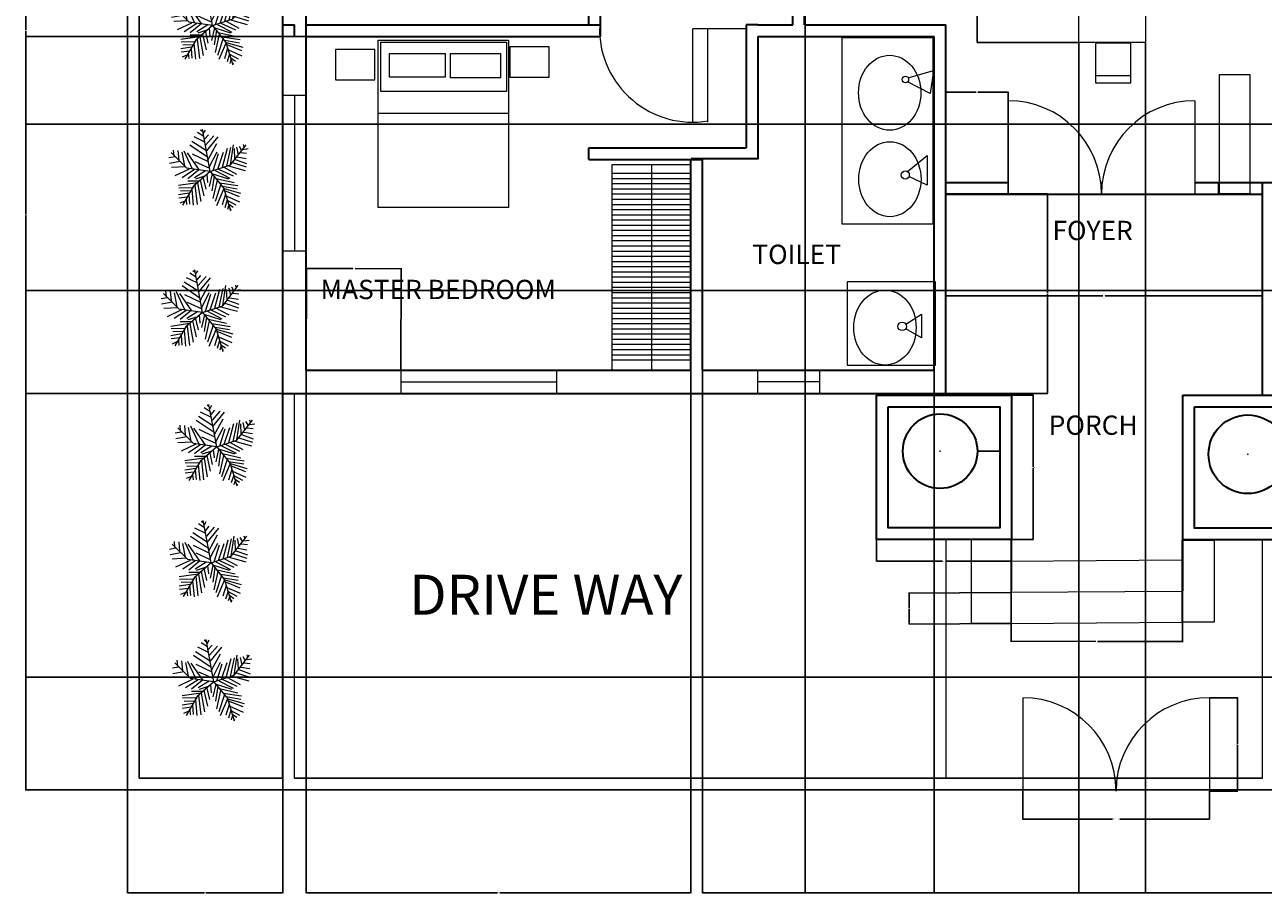
# Model space of a CAD drawing. Units: inches. Extents: x -86 to 773, y -188 to 560.
# Tile 1 of 6: x -86 to 392, y -188 to 147. Entities that reach past the tile are written whole.
import ezdxf

# ---------------------------------------------------------------- set-up
doc = ezdxf.new("R2010")
doc.units = ezdxf.units.IN
doc.header["$MEASUREMENT"] = 0
for name, color, linetype, lineweight in [('A-ANNO-DIMS', 2, 'Continuous', 18), ('A-AREA-IDEN', 7, 'Continuous', 25), ('A-COLS', 7, 'Continuous', 35), ('A-DOOR', 7, 'Continuous', 18), ('A-FLOR-FIXT', 8, 'Continuous', 18), ('A-FLOR-STRS', 7, 'Continuous', 18), ('A-FURN', 8, 'Continuous', 18), ('A-FURN-PATT', 8, 'Continuous', 9), ('A-GLAZ', 7, 'Continuous', 18), ('A-WALL', 7, 'Continuous', 35), ('C-PROP', 7, 'Continuous', 25), ('L-HRDS', 7, 'Continuous', 18), ('L-PLNT-TREE', 8, 'Continuous', 9)]:
    doc.layers.add(name, color=color, linetype=linetype, lineweight=lineweight)
doc.styles.get("Standard").update_dxf_attribs({"font": 'arial.ttf'})
doc.dimstyles.get("Standard").update_dxf_attribs({"dimtxt": 0.18, "dimasz": 0.18, "dimexe": 0.18, "dimexo": 0.0625, "dimgap": 0.09, "dimtad": 0, "dimtih": 1, "dimtoh": 1, "dimdec": 4, "dimzin": 0, "dimdsep": 46, "dimtxsty": 'Standard', "dimcen": 0.09, "dimadec": 0, "dimazin": 0, "dimtfac": 1, "dimtdec": 4, "dimtofl": 0, "dimtmove": 0, "dimatfit": 3, "dimfxl": 1, "dimtolj": 1, "dimtzin": 0, "dimarcsym": 0})

# ---------------------------------------------------------------- blocks, each defined once
blk = doc.blocks.new('Trees - Metric')
for p, q in [((-221.9198, 1197.3052), (-433.5526, 1338.8594)), ((-258.7244, 1362.456), (-332.3336, 1421.4348)), ((0, 0), (-266.7, 1447.8)), ((-231.1146, 1315.2628), (-166.7002, 1421.4348)), ((-93.091, 489.5342), (-700.3796, 902.3858)), ((-129.8956, 713.6638), (-626.7704, 1032.1544)), ((-185.1152, 1008.5578), (-553.1612, 1185.4942)), ((-194.31, 1102.9442), (-65.4812, 1256.284)), ((-148.3106, 914.1968), (118.5418, 1220.9018)), ((-129.8956, 701.8528), (265.7602, 1185.4942)), ((-74.7014, 418.7444), (219.7608, 961.39)), ((685.8, 228.6), (1219.2, 914.4)), ((689.0258, 230.0224), (790.2448, 914.1968)), ((983.4626, 867.0036), (1066.2666, 725.4494)), ((1121.4862, 925.9824), (1149.0706, 831.6214)), ((-1206.4492, 501.3198), (-1418.082, 465.9376)), ((-800.1, 114.3), (-1333.5, 647.7)), ((-1234.059, 536.7274), (-1252.4486, 737.2604)), ((-1105.2302, 725.4494), (-1077.6458, 395.1732)), ((-976.4268, 666.4706), (-884.4026, 194.6402)), ((-902.8176, 713.6638), (-617.5756, 100.2538)), ((-369.1382, 53.086), (-783.1836, 642.874)), ((-617.5756, 607.4918), (-74.7014, 347.98)), ((-28.6766, 171.0436), (228.9556, 678.2816)), ((100.1268, 41.275), (284.1498, 619.2774)), ((256.5654, 88.4682), (449.7832, 666.4706)), ((412.9786, 147.447), (587.8068, 796.2392)), ((560.197, 182.8292), (698.2206, 819.8358)), ((808.6344, 784.4282), (827.0494, 418.7444)), ((891.4384, 831.6214), (946.658, 572.1096)), ((919.0482, 501.3198), (1222.6798, 454.152)), ((1029.462, 654.685), (1241.0948, 631.0884)), ((1112.2914, 760.8316), (1296.3144, 784.4282)), ((-1031.621, 347.98), (-1399.667, 277.1902)), ((-847.598, 159.2326), (-1326.0578, 135.636)), ((-718.7946, 88.4682), (-1215.644, -147.447)), ((-543.9664, 76.6572), (-967.2066, -206.4512)), ((0, 0), (-800.1, 114.3)), ((-405.9428, 53.086), (-764.794, -241.8334)), ((0, 0), (-571.5, -495.3)), ((-166.7002, 29.4894), (-543.9664, -206.4512)), ((-525.5514, 347.98), (-28.6766, 123.8504)), ((0, 0), (685.8, 228.6)), ((0, 0), (457.2, -571.5)), ((164.5412, 41.275), (661.416, -218.2368)), ((284.1498, 88.4682), (781.0246, -147.447)), ((458.978, 147.447), (891.4384, -88.4682)), ((615.4166, 194.6402), (1185.8752, 41.275)), ((753.4148, 312.5978), (1222.6798, 159.2326)), ((845.439, 418.7444), (1241.0948, 277.1902)), ((-442.7474, -383.3876), (-1086.8406, -477.7486)), ((-387.5278, -324.4088), (-764.794, -324.4088)), ((-166.7002, -147.447), (-507.1618, -253.619)), ((-433.5526, -383.3876), (-323.1134, -1020.3688)), ((-341.5284, -289.0012), (-221.9198, -831.6214)), ((-240.3094, -218.2368), (-157.5054, -595.7062)), ((-120.7008, -88.4682), (-93.091, -371.5766)), ((63.3222, -76.6826), (-37.8714, -513.1308)), ((44.9326, -64.897), (615.4166, -241.8334)), ((127.7366, -159.258), (54.1274, -654.685)), ((228.9556, -289.0012), (90.932, -914.1968)), ((192.151, -230.0224), (817.8292, -371.5766)), ((311.7596, -383.3876), (937.4378, -477.7486)), ((-718.7946, -737.2604), (-1086.8406, -796.2392)), ((-617.5756, -548.5384), (-1077.6458, -560.324)), ((-681.9646, -666.496), (-1022.4262, -654.685)), ((-571.5, -495.3), (-952.5, -1143)), ((-737.1842, -784.4536), (-709.5744, -1114.7298)), ((-635.9652, -607.5172), (-580.771, -1150.1374)), ((-525.5514, -465.963), (-451.9422, -1126.5408)), ((357.759, -430.5554), (164.5412, -1020.3688)), ((458.978, -572.1096), (210.5406, -1161.923)), ((514.1976, -772.6426), (403.7838, -1138.3264)), ((412.9786, -501.3452), (919.0482, -583.9206)), ((457.2, -571.5), (685.8, -1333.5)), ((468.1982, -572.1096), (1029.462, -737.2604)), ((486.5878, -642.8994), (983.4626, -843.4324)), ((541.8074, -831.6214), (992.6574, -1032.1544)), ((-783.1836, -867.029), (-1077.6458, -902.4112)), ((-875.2078, -1008.5832), (-1040.8412, -1079.3476)), ((-829.2084, -937.7934), (-810.7934, -1126.5408)), ((578.612, -961.39), (495.7826, -1232.7128)), ((578.612, -973.1756), (873.0488, -1138.3264)), ((624.6114, -1161.923), (587.8068, -1291.6916)), ((624.6114, -1102.9442), (781.0246, -1209.1162)), ((679.8056, -1268.095), (716.6102, -1291.6916))]:
    blk.add_line(p, q)
blk = doc.blocks.new('BED-DOUBLE-NIGHTSTANDS')
blk.add_line((16.69, 36.48), (66.76, 36.48))
for points in [[(16.43, 64.62), (66.76, 64.62), (66.76, 0), (16.43, 0)], [(17.47, 63.83), (65.98, 63.83), (65.98, 44.81), (17.47, 44.81)], [(15.13, 60.97), (0, 60.97), (0, 49.24), (15.13, 49.24)], [(20.86, 59.41), (42.25, 59.41), (42.25, 50.29), (20.86, 50.29)], [(44.34, 59.41), (63.63, 59.41), (63.63, 50.03), (44.34, 50.03)], [(82.41, 62.01), (67.29, 62.01), (67.29, 50.29), (82.41, 50.29)]]:
    blk.add_lwpolyline(points, close=True)
blk = doc.blocks.new('DOOR-DOUBLE-72')
for p, q in [((0, 36), (0, 0)), ((72, 36), (72, 0))]:
    blk.add_line(p, q)
for centre, start, end in [((0, 0), 0, 90), ((72, 0), 90, 180)]:
    blk.add_arc(centre, 36, start, end)
blk = doc.blocks.new('WIN-60-W9')
for p, q in [((0, 60), (9, 60)), ((4.5, 60), (4.5, 0)), ((0, 0), (9, 0))]:
    blk.add_line(p, q)
blk = doc.blocks.new('WIN-24-W9')
for p, q in [((0, 9), (0, 0)), ((24, 9), (24, 0)), ((24, 4.5), (0, 4.5))]:
    blk.add_line(p, q)
blk = doc.blocks.new('DINING-CHAIR')
blk.add_line((0, 12.55), (13.8, 12.55))
blk.add_lwpolyline([(0.02, 0), (13.65, 0), (13.65, 15.22), (0.02, 15.22)], close=True)
blk = doc.blocks.new('BASIN-TAP')
blk.add_lwpolyline([(3.11, 5.27), (9.09, 9.11), (9.09, 0), (3.06, 3.55)])
blk.add_circle((1.66, 4.45), 1.66)
blk = doc.blocks.new('PORCH-COLUMN-PLINTH')
for points in [[(0, 55.74), (51.99, 55.74), (51.99, 0), (0, 0)], [(4.5, 51.24), (47.49, 51.24), (47.49, 4.5), (4.5, 4.5)]]:
    blk.add_lwpolyline(points, close=True)
blk = doc.blocks.new('*D33')
at = {"layer": 'A-ANNO-DIMS', "color": 0, "lineweight": -2, "transparency": 16777216}
for p, q in [((299.01, -148.39), (299.01, -159.31)), ((371.01, -148.39), (371.01, -159.31)), ((299.19, -159.13), (333.59, -159.13)), ((370.83, -159.13), (336.44, -159.13))]:
    blk.add_line(p, q, dxfattribs=at)
at = {"layer": 'A-ANNO-DIMS', "color": 0, "transparency": 16777216}
for points in [[(299.19, -159.1), (299.19, -159.16), (299.01, -159.13)], [(370.83, -159.1), (370.83, -159.16), (371.01, -159.13)]]:
    blk.add_solid(points, dxfattribs=at)
at = {"layer": 'Defpoints', "color": 0, "transparency": 16777216}
for p in [(299.01, -148.33), (371.01, -148.33), (371.01, -159.13)]:
    blk.add_point(p, dxfattribs=at)
at = {"layer": 'A-ANNO-DIMS', "color": 0, "transparency": 16777216, "insert": (335.01, -159.13), "char_height": 0.18, "attachment_point": 5}
blk.add_mtext('\\A1;DOUBLE LEAF 72 TYP.', dxfattribs=at)
blk = doc.blocks.new('*D34')
at = {"layer": 'A-ANNO-DIMS', "color": 0, "lineweight": -2, "transparency": 16777216}
for p, q in [((371.08, -112.33), (381.99, -112.33)), ((381.81, -112.51), (381.81, -130.15)), ((381.81, -148.15), (381.81, -130.51)), ((371.08, -148.33), (381.99, -148.33))]:
    blk.add_line(p, q, dxfattribs=at)
at = {"layer": 'A-ANNO-DIMS', "color": 0, "transparency": 16777216}
for points in [[(381.78, -112.51), (381.84, -112.51), (381.81, -112.33)], [(381.78, -148.15), (381.84, -148.15), (381.81, -148.33)]]:
    blk.add_solid(points, dxfattribs=at)
at = {"layer": 'Defpoints', "color": 0, "transparency": 16777216}
for p in [(371.01, -112.33), (381.81, -112.33), (371.01, -148.33)]:
    blk.add_point(p, dxfattribs=at)
at = {"layer": 'A-ANNO-DIMS', "color": 0, "transparency": 16777216, "insert": (381.81, -130.33), "char_height": 0.18, "attachment_point": 5}
blk.add_mtext('\\A1;36 TYP.', dxfattribs=at)
blk = doc.blocks.new('*D43')
at = {"layer": 'A-ANNO-DIMS', "color": 0, "lineweight": -2, "transparency": 16777216}
for p, q in [((294.66, 4.44), (303.14, 4.44)), ((302.96, 4.26), (302.96, -23.25)), ((302.96, -51.12), (302.96, -23.61)), ((294.66, -51.3), (303.14, -51.3))]:
    blk.add_line(p, q, dxfattribs=at)
at = {"layer": 'A-ANNO-DIMS', "color": 0, "transparency": 16777216}
for points in [[(302.93, 4.26), (302.99, 4.26), (302.96, 4.44)], [(302.93, -51.12), (302.99, -51.12), (302.96, -51.3)]]:
    blk.add_solid(points, dxfattribs=at)
at = {"layer": 'Defpoints', "color": 0, "transparency": 16777216}
for p in [(294.6, 4.44), (302.96, 4.44), (294.6, -51.3)]:
    blk.add_point(p, dxfattribs=at)
at = {"layer": 'A-ANNO-DIMS', "color": 0, "transparency": 16777216, "insert": (302.96, -23.43), "char_height": 0.18, "attachment_point": 5}
blk.add_mtext('\\A1;PLINTH 56 TYP.', dxfattribs=at)
blk = doc.blocks.new('*D44')
at = {"layer": 'A-ANNO-DIMS', "color": 0, "lineweight": -2, "transparency": 16777216}
for p, q in [((242.61, -51.36), (242.61, -59.84)), ((294.6, -51.36), (294.6, -59.84)), ((242.79, -59.66), (268.07, -59.66)), ((294.42, -59.66), (269.13, -59.66))]:
    blk.add_line(p, q, dxfattribs=at)
at = {"layer": 'A-ANNO-DIMS', "color": 0, "transparency": 16777216}
for points in [[(242.79, -59.63), (242.79, -59.69), (242.61, -59.66)], [(294.42, -59.63), (294.42, -59.69), (294.6, -59.66)]]:
    blk.add_solid(points, dxfattribs=at)
at = {"layer": 'Defpoints', "color": 0, "transparency": 16777216}
for p in [(242.61, -51.3), (294.6, -51.3), (294.6, -59.66)]:
    blk.add_point(p, dxfattribs=at)
at = {"layer": 'A-ANNO-DIMS', "color": 0, "transparency": 16777216, "insert": (268.6, -59.66), "char_height": 0.18, "attachment_point": 5}
blk.add_mtext('\\A1;52 TYP.', dxfattribs=at)
blk = doc.blocks.new('*D47')
at = {"layer": 'A-ANNO-DIMS', "color": 0, "lineweight": -2, "transparency": 16777216}
for p, q in [((-46.55, -147.98), (-46.55, -187.76)), ((13.45, -143.48), (13.45, -187.76)), ((-46.37, -187.58), (-16.77, -187.58)), ((13.27, -187.58), (-16.33, -187.58))]:
    blk.add_line(p, q, dxfattribs=at)
at = {"layer": 'A-ANNO-DIMS', "color": 0, "transparency": 16777216}
for points in [[(-46.37, -187.55), (-46.37, -187.61), (-46.55, -187.58)], [(13.27, -187.55), (13.27, -187.61), (13.45, -187.58)]]:
    blk.add_solid(points, dxfattribs=at)
at = {"layer": 'Defpoints', "color": 0, "transparency": 16777216}
for p in [(-46.55, -147.92), (13.45, -143.42), (13.45, -187.58)]:
    blk.add_point(p, dxfattribs=at)
at = {"layer": 'A-ANNO-DIMS', "color": 0, "transparency": 16777216, "insert": (-16.55, -187.58), "char_height": 0.18, "attachment_point": 5}
blk.add_mtext('\\A1;60', dxfattribs=at)
blk = doc.blocks.new('*D49')
at = {"layer": 'A-ANNO-DIMS', "color": 0, "lineweight": -2, "transparency": 16777216}
for p, q in [((13.39, 5.02), (-85.98, 5.02)), ((-85.8, 4.84), (-85.8, -71.27)), ((-85.8, -147.74), (-85.8, -71.63)), ((-46.61, -147.92), (-85.98, -147.92))]:
    blk.add_line(p, q, dxfattribs=at)
at = {"layer": 'A-ANNO-DIMS', "color": 0, "transparency": 16777216}
for points in [[(-85.83, 4.84), (-85.77, 4.84), (-85.8, 5.02)], [(-85.83, -147.74), (-85.77, -147.74), (-85.8, -147.92)]]:
    blk.add_solid(points, dxfattribs=at)
at = {"layer": 'Defpoints', "color": 0, "transparency": 16777216}
for p in [(-85.8, 5.02), (13.45, 5.02), (-46.55, -147.92)]:
    blk.add_point(p, dxfattribs=at)
at = {"layer": 'A-ANNO-DIMS', "color": 0, "transparency": 16777216, "insert": (-85.8, -71.45), "char_height": 0.18, "attachment_point": 5}
blk.add_mtext('\\A1;152.94', dxfattribs=at)
blk = doc.blocks.new('*D50')
at = {"layer": 'A-ANNO-DIMS', "color": 0, "lineweight": -2, "transparency": 16777216}
for p, q in [((22.39, 142.78), (-85.98, 142.78)), ((-85.8, 142.6), (-85.8, 74.08)), ((-85.8, 5.2), (-85.8, 73.72)), ((13.39, 5.02), (-85.98, 5.02))]:
    blk.add_line(p, q, dxfattribs=at)
at = {"layer": 'A-ANNO-DIMS', "color": 0, "transparency": 16777216}
for points in [[(-85.83, 142.6), (-85.77, 142.6), (-85.8, 142.78)], [(-85.83, 5.2), (-85.77, 5.2), (-85.8, 5.02)]]:
    blk.add_solid(points, dxfattribs=at)
at = {"layer": 'Defpoints', "color": 0, "transparency": 16777216}
for p in [(-85.8, 142.78), (22.45, 142.78), (13.45, 5.02)]:
    blk.add_point(p, dxfattribs=at)
at = {"layer": 'A-ANNO-DIMS', "color": 0, "transparency": 16777216, "insert": (-85.8, 73.9), "char_height": 0.18, "attachment_point": 5}
blk.add_mtext('\\A1;137.76', dxfattribs=at)
blk = doc.blocks.new('*D53')
at = {"layer": 'A-ANNO-DIMS', "color": 0, "lineweight": -2, "transparency": 16777216}
for p, q in [((623.74, 44.83), (-85.98, 44.83)), ((-85.8, 44.65), (-85.8, -29.62)), ((-85.8, -104.26), (-85.8, -29.99)), ((623.93, -104.44), (-85.98, -104.44))]:
    blk.add_line(p, q, dxfattribs=at)
at = {"layer": 'A-ANNO-DIMS', "color": 0, "transparency": 16777216}
for points in [[(-85.83, 44.65), (-85.77, 44.65), (-85.8, 44.83)], [(-85.83, -104.26), (-85.77, -104.26), (-85.8, -104.44)]]:
    blk.add_solid(points, dxfattribs=at)
at = {"layer": 'Defpoints', "color": 0, "transparency": 16777216}
for p in [(623.81, 44.83), (-85.8, -104.44), (623.99, -104.44)]:
    blk.add_point(p, dxfattribs=at)
at = {"layer": 'A-ANNO-DIMS', "color": 0, "transparency": 16777216, "insert": (-85.8, -29.81), "char_height": 0.18, "attachment_point": 5}
blk.add_mtext('\\A1;149.27', dxfattribs=at)
blk = doc.blocks.new('*D63')
at = {"layer": 'A-ANNO-DIMS', "color": 0, "lineweight": -2, "transparency": 16777216}
for p, q in [((22.45, 13.96), (22.45, -187.76)), ((170.89, 13.96), (170.89, -187.76)), ((22.63, -187.58), (96.22, -187.58)), ((170.71, -187.58), (97.13, -187.58))]:
    blk.add_line(p, q, dxfattribs=at)
at = {"layer": 'A-ANNO-DIMS', "color": 0, "transparency": 16777216}
for points in [[(22.63, -187.55), (22.63, -187.61), (22.45, -187.58)], [(170.71, -187.55), (170.71, -187.61), (170.89, -187.58)]]:
    blk.add_solid(points, dxfattribs=at)
at = {"layer": 'Defpoints', "color": 0, "transparency": 16777216}
for p in [(22.45, 14.02), (170.89, 14.02), (170.89, -187.58)]:
    blk.add_point(p, dxfattribs=at)
at = {"layer": 'A-ANNO-DIMS', "color": 0, "transparency": 16777216, "insert": (96.67, -187.58), "char_height": 0.18, "attachment_point": 5}
blk.add_mtext('\\A1;148.44', dxfattribs=at)
blk = doc.blocks.new('*D64')
at = {"layer": 'A-ANNO-DIMS', "color": 0, "lineweight": -2, "transparency": 16777216}
for p, q in [((175.39, 13.96), (175.39, -187.76)), ((264.79, 13.96), (264.79, -187.76)), ((175.57, -187.58), (219.77, -187.58)), ((264.61, -187.58), (220.42, -187.58))]:
    blk.add_line(p, q, dxfattribs=at)
at = {"layer": 'A-ANNO-DIMS', "color": 0, "transparency": 16777216}
for points in [[(175.57, -187.55), (175.57, -187.61), (175.39, -187.58)], [(264.61, -187.55), (264.61, -187.61), (264.79, -187.58)]]:
    blk.add_solid(points, dxfattribs=at)
at = {"layer": 'Defpoints', "color": 0, "transparency": 16777216}
for p in [(175.39, 14.02), (264.79, 14.02), (264.79, -187.58)]:
    blk.add_point(p, dxfattribs=at)
at = {"layer": 'A-ANNO-DIMS', "color": 0, "transparency": 16777216, "insert": (220.09, -187.58), "char_height": 0.18, "attachment_point": 5}
blk.add_mtext('\\A1;89.4', dxfattribs=at)
blk = doc.blocks.new('*D65')
at = {"layer": 'A-ANNO-DIMS', "color": 0, "lineweight": -2, "transparency": 16777216}
for p, q in [((446.53, 366.45), (446.53, -187.76)), ((215.06, 361.95), (215.06, -187.76)), ((215.24, -187.58), (330.33, -187.58)), ((446.35, -187.58), (331.26, -187.58))]:
    blk.add_line(p, q, dxfattribs=at)
at = {"layer": 'A-ANNO-DIMS', "color": 0, "transparency": 16777216}
for points in [[(215.24, -187.55), (215.24, -187.61), (215.06, -187.58)], [(446.35, -187.55), (446.35, -187.61), (446.53, -187.58)]]:
    blk.add_solid(points, dxfattribs=at)
at = {"layer": 'Defpoints', "color": 0, "transparency": 16777216}
for p in [(446.53, 366.52), (215.06, 362.02), (446.53, -187.58)]:
    blk.add_point(p, dxfattribs=at)
at = {"layer": 'A-ANNO-DIMS', "color": 0, "transparency": 16777216, "insert": (330.8, -187.58), "char_height": 0.18, "attachment_point": 5}
blk.add_mtext('\\A1;231.47', dxfattribs=at)
blk = doc.blocks.new('*D66')
at = {"layer": 'A-ANNO-DIMS', "color": 0, "lineweight": -2, "transparency": 16777216}
for p, q in [((269.29, 81.93), (269.29, 42.57)), ((391.47, 81.93), (391.47, 42.57)), ((269.47, 42.75), (329.92, 42.75)), ((391.29, 42.75), (330.83, 42.75))]:
    blk.add_line(p, q, dxfattribs=at)
at = {"layer": 'A-ANNO-DIMS', "color": 0, "transparency": 16777216}
for points in [[(269.47, 42.78), (269.47, 42.72), (269.29, 42.75)], [(391.29, 42.78), (391.29, 42.72), (391.47, 42.75)]]:
    blk.add_solid(points, dxfattribs=at)
at = {"layer": 'Defpoints', "color": 0, "transparency": 16777216}
for p in [(269.29, 82), (391.47, 82), (269.29, 42.75)]:
    blk.add_point(p, dxfattribs=at)
at = {"layer": 'A-ANNO-DIMS', "color": 0, "transparency": 16777216, "insert": (330.38, 42.75), "char_height": 0.18, "attachment_point": 5}
blk.add_mtext('\\A1;122.17', dxfattribs=at)
blk = doc.blocks.new('*D73')
at = {"layer": 'A-ANNO-DIMS', "color": 0, "lineweight": -2, "transparency": 16777216}
for p, q in [((577.4, 181.27), (-85.98, 181.27)), ((-85.8, 181.09), (-85.8, 145.29)), ((-85.8, 109.12), (-85.8, 144.92)), ((577.4, 108.94), (-85.98, 108.94))]:
    blk.add_line(p, q, dxfattribs=at)
at = {"layer": 'A-ANNO-DIMS', "color": 0, "transparency": 16777216}
for points in [[(-85.83, 181.09), (-85.77, 181.09), (-85.8, 181.27)], [(-85.83, 109.12), (-85.77, 109.12), (-85.8, 108.94)]]:
    blk.add_solid(points, dxfattribs=at)
at = {"layer": 'Defpoints', "color": 0, "transparency": 16777216}
for p in [(-85.8, 181.27), (577.46, 181.27), (577.46, 108.94)]:
    blk.add_point(p, dxfattribs=at)
at = {"layer": 'A-ANNO-DIMS', "color": 0, "transparency": 16777216, "insert": (-85.8, 145.11), "char_height": 0.18, "attachment_point": 5}
blk.add_mtext('\\A1;72.33', dxfattribs=at)
blk = doc.blocks.new('*D77')
at = {"layer": 'A-ANNO-DIMS', "color": 0, "lineweight": -2, "transparency": 16777216}
for p, q in [((320.69, 140.33), (320.69, -187.76)), ((346.35, 140.33), (346.35, -187.76)), ((320.87, -187.58), (333.13, -187.58)), ((346.17, -187.58), (333.92, -187.58))]:
    blk.add_line(p, q, dxfattribs=at)
at = {"layer": 'A-ANNO-DIMS', "color": 0, "transparency": 16777216}
for points in [[(320.87, -187.55), (320.87, -187.61), (320.69, -187.58)], [(346.17, -187.55), (346.17, -187.61), (346.35, -187.58)]]:
    blk.add_solid(points, dxfattribs=at)
at = {"layer": 'Defpoints', "color": 0, "transparency": 16777216}
for p in [(320.69, 140.39), (346.35, 140.39), (346.35, -187.58)]:
    blk.add_point(p, dxfattribs=at)
at = {"layer": 'A-ANNO-DIMS', "color": 0, "transparency": 16777216, "insert": (333.52, -187.58), "char_height": 0.18, "attachment_point": 5}
blk.add_mtext('\\A1;25.66', dxfattribs=at)
blk = doc.blocks.new('*D78')
at = {"layer": 'A-ANNO-DIMS', "color": 0, "lineweight": -2, "transparency": 16777216}
for p, q in [((320.63, 194.07), (281.26, 194.07)), ((281.44, 193.89), (281.44, 167.41)), ((281.44, 140.57), (281.44, 167.05)), ((320.63, 140.39), (281.26, 140.39))]:
    blk.add_line(p, q, dxfattribs=at)
at = {"layer": 'A-ANNO-DIMS', "color": 0, "transparency": 16777216}
for points in [[(281.41, 193.89), (281.47, 193.89), (281.44, 194.07)], [(281.41, 140.57), (281.47, 140.57), (281.44, 140.39)]]:
    blk.add_solid(points, dxfattribs=at)
at = {"layer": 'Defpoints', "color": 0, "transparency": 16777216}
for p in [(281.44, 194.07), (320.69, 194.07), (320.69, 140.39)]:
    blk.add_point(p, dxfattribs=at)
at = {"layer": 'A-ANNO-DIMS', "color": 0, "transparency": 16777216, "insert": (281.44, 167.23), "char_height": 0.18, "attachment_point": 5}
blk.add_mtext('\\A1;53.68', dxfattribs=at)
blk = doc.blocks.new('*D82')
at = {"layer": 'A-ANNO-DIMS', "color": 0, "lineweight": -2, "transparency": 16777216}
for p, q in [((269.35, 82), (308.72, 82)), ((308.54, 81.82), (308.54, 43.69)), ((308.54, 5.2), (308.54, 43.33)), ((269.35, 5.02), (308.72, 5.02))]:
    blk.add_line(p, q, dxfattribs=at)
at = {"layer": 'A-ANNO-DIMS', "color": 0, "transparency": 16777216}
for points in [[(308.51, 81.82), (308.57, 81.82), (308.54, 82)], [(308.51, 5.2), (308.57, 5.2), (308.54, 5.02)]]:
    blk.add_solid(points, dxfattribs=at)
at = {"layer": 'Defpoints', "color": 0, "transparency": 16777216}
for p in [(269.29, 82), (269.29, 5.02), (308.54, 5.02)]:
    blk.add_point(p, dxfattribs=at)
at = {"layer": 'A-ANNO-DIMS', "color": 0, "transparency": 16777216, "insert": (308.54, 43.51), "char_height": 0.18, "attachment_point": 5}
blk.add_mtext('\\A1;76.97', dxfattribs=at)
blk = doc.blocks.new('*D83')
at = {"layer": 'A-ANNO-DIMS', "color": 0, "lineweight": -2, "transparency": 16777216}
for p, q in [((269.29, 82.06), (269.3, 121.43)), ((269.48, 121.25), (281.04, 121.25)), ((293.21, 121.24), (281.65, 121.25)), ((293.39, 82.06), (293.39, 121.42))]:
    blk.add_line(p, q, dxfattribs=at)
at = {"layer": 'A-ANNO-DIMS', "color": 0, "transparency": 16777216}
for points in [[(269.48, 121.28), (269.48, 121.22), (269.3, 121.25)], [(293.21, 121.27), (293.21, 121.21), (293.39, 121.24)]]:
    blk.add_solid(points, dxfattribs=at)
at = {"layer": 'Defpoints', "color": 0, "transparency": 16777216}
for p in [(293.39, 121.24), (269.29, 82), (293.39, 81.99)]:
    blk.add_point(p, dxfattribs=at)
at = {"layer": 'A-ANNO-DIMS', "color": 0, "transparency": 16777216, "insert": (281.35, 121.25), "char_height": 0.18, "attachment_point": 5}
blk.add_mtext('\\A1;24.1', dxfattribs=at)
blk = doc.blocks.new('*D84')
at = {"layer": 'A-ANNO-DIMS', "color": 0, "lineweight": -2, "transparency": 16777216}
for p, q in [((294.6, -51.36), (294.53, -90.73)), ((360.76, -51.47), (360.69, -90.84)), ((294.71, -90.55), (327.22, -90.6)), ((360.51, -90.66), (328, -90.6))]:
    blk.add_line(p, q, dxfattribs=at)
at = {"layer": 'A-ANNO-DIMS', "color": 0, "transparency": 16777216}
for points in [[(294.71, -90.52), (294.71, -90.58), (294.53, -90.55)], [(360.51, -90.63), (360.51, -90.69), (360.69, -90.66)]]:
    blk.add_solid(points, dxfattribs=at)
at = {"layer": 'Defpoints', "color": 0, "transparency": 16777216}
for p in [(294.6, -51.3), (360.76, -51.41), (294.53, -90.55)]:
    blk.add_point(p, dxfattribs=at)
at = {"layer": 'A-ANNO-DIMS', "color": 0, "transparency": 16777216, "insert": (327.61, -90.6), "char_height": 0.18, "attachment_point": 5}
blk.add_mtext('\\A1;66.17', dxfattribs=at)
blk = doc.blocks.new('*D85')
at = {"layer": 'A-ANNO-DIMS', "color": 0, "lineweight": -2, "transparency": 16777216}
for p, q in [((294.27, -71.68), (254.91, -71.96)), ((255.09, -72.14), (255.13, -77.78)), ((255.17, -83.78), (255.13, -78.14)), ((294.36, -83.68), (254.99, -83.96))]:
    blk.add_line(p, q, dxfattribs=at)
at = {"layer": 'A-ANNO-DIMS', "color": 0, "transparency": 16777216}
for points in [[(255.12, -72.14), (255.06, -72.14), (255.09, -71.96)], [(255.2, -83.78), (255.14, -83.78), (255.17, -83.96)]]:
    blk.add_solid(points, dxfattribs=at)
at = {"layer": 'Defpoints', "color": 0, "transparency": 16777216}
for p in [(294.34, -71.68), (255.09, -71.96), (294.42, -83.68)]:
    blk.add_point(p, dxfattribs=at)
at = {"layer": 'A-ANNO-DIMS', "color": 0, "transparency": 16777216, "insert": (255.13, -77.96), "char_height": 0.18, "attachment_point": 5}
blk.add_mtext('\\A1;12', dxfattribs=at)
blk = doc.blocks.new('*D86')
at = {"layer": 'A-ANNO-DIMS', "color": 0, "lineweight": -2, "transparency": 16777216}
for p, q in [((22.45, 14.09), (22.58, 53.45)), ((22.76, 53.27), (40.4, 53.22)), ((58.97, 53.16), (41.33, 53.21)), ((59.03, 13.97), (59.15, 53.34))]:
    blk.add_line(p, q, dxfattribs=at)
at = {"layer": 'A-ANNO-DIMS', "color": 0, "transparency": 16777216}
for points in [[(22.76, 53.3), (22.76, 53.24), (22.58, 53.27)], [(58.97, 53.19), (58.97, 53.13), (59.15, 53.16)]]:
    blk.add_solid(points, dxfattribs=at)
at = {"layer": 'Defpoints', "color": 0, "transparency": 16777216}
for p in [(59.15, 53.16), (22.45, 14.02), (59.03, 13.91)]:
    blk.add_point(p, dxfattribs=at)
at = {"layer": 'A-ANNO-DIMS', "color": 0, "transparency": 16777216, "insert": (40.86, 53.21), "char_height": 0.18, "attachment_point": 5}
blk.add_mtext('\\A1;36.576', dxfattribs=at)
blk = doc.blocks.new('*D91')
at = {"layer": 'A-ANNO-DIMS', "color": 0, "lineweight": -2, "transparency": 16777216}
for p, q in [((267, -17.23), (267.18, -17.23)), ((267.09, -17.32), (267.09, -17.14)), ((290.1, -17.22), (281.65, -17.23))]:
    blk.add_line(p, q, dxfattribs=at)
at = {"layer": 'A-ANNO-DIMS', "color": 0, "transparency": 16777216}
blk.add_solid([(281.65, -17.19), (281.65, -17.25), (281.47, -17.23)], dxfattribs=at)
at = {"layer": 'Defpoints', "color": 0, "transparency": 16777216}
for p in [(252.7, -17.23), (281.47, -17.23)]:
    blk.add_point(p, dxfattribs=at)
at = {"layer": 'A-ANNO-DIMS', "color": 0, "transparency": 16777216, "insert": (290.6, -17.22), "char_height": 0.18, "attachment_point": 5}
blk.add_mtext('\\A1;∅28.77', dxfattribs=at)
blk = doc.blocks.new('*D92')
at = {"layer": 'A-ANNO-DIMS', "color": 0, "lineweight": -2, "transparency": 16777216}
for p, q in [((385.79, -18.42), (385.97, -18.42)), ((385.88, -18.51), (385.88, -18.33)), ((410.18, -18.42), (401.25, -18.42))]:
    blk.add_line(p, q, dxfattribs=at)
at = {"layer": 'A-ANNO-DIMS', "color": 0, "transparency": 16777216}
blk.add_solid([(401.25, -18.39), (401.25, -18.45), (401.07, -18.42)], dxfattribs=at)
at = {"layer": 'Defpoints', "color": 0, "transparency": 16777216}
for p in [(370.7, -18.42), (401.07, -18.42)]:
    blk.add_point(p, dxfattribs=at)
at = {"layer": 'A-ANNO-DIMS', "color": 0, "transparency": 16777216, "insert": (410.67, -18.42), "char_height": 0.18, "attachment_point": 5}
blk.add_mtext('\\A1;∅30.37', dxfattribs=at)

msp = doc.modelspace()

# ---------------------------------------------------------------- hatches: boundary and pattern name
at = {"layer": 'A-FURN-PATT'}
h = msp.add_hatch(dxfattribs=at)
h.set_pattern_fill('ANSI31', color=256, scale=16, angle=-45, style=0)
h.paths.add_polyline_path([(140.4677, 17.1086), (170.8915, 17.1086), (170.8915, 91.1086), (140.4677, 91.1086)])

# ---------------------------------------------------------------- linework, layer by layer
at = {"layer": 'A-COLS'}
for centre, radius in [((267.0859, -17.2254), 14.3861), ((385.883, -18.4243), 15.1853)]:
    msp.add_circle(centre, radius, dxfattribs=at)
at = {"layer": 'A-DOOR'}
for p, q in [((136.0315, 145.7001), (135.6243, 145.7001)), ((192.3054, 145.7001), (171.6051, 145.7001)), ((171.6051, 109.7001), (171.6051, 145.7001)), ((171.6243, 109.7001), (171.6243, 145.7001)), ((177.438, 109.7001), (177.438, 145.7001))]:
    msp.add_line(p, q, dxfattribs=at)
msp.add_arc((171.6243, 145.7001), 36, 180, 279.293446, dxfattribs=at)
at = {"layer": 'A-FLOR-FIXT'}
for points in [[(229.262, 142.3304), (264.2811, 142.3304), (264.2811, 70.3929), (229.262, 70.3929)], [(231.2765, 16.015), (265.2725, 16.015), (265.2725, 48.092), (231.2765, 48.092)]]:
    msp.add_lwpolyline(points, close=True, dxfattribs=at)
for points in [[(254.7697, 126.8173), (264.5145, 129.7019), (263.2945, 120.7641), (254.5742, 125.3095)], [(254.4898, 90.6604), (262.0746, 96.7947), (262.0746, 85.4194), (255.0869, 88.7262)]]:
    msp.add_lwpolyline(points, dxfattribs=at)
for centre, radius in [((253.6987, 126.1895), 1.2414), ((253.6475, 89.3411), 1.5652)]:
    msp.add_circle(centre, radius, dxfattribs=at)
for centre in [(247.6449, 121.0515), (247.7109, 87.7166), (245.8222, 30.4811)]:
    msp.add_ellipse(centre, major_axis=(0, 14.4661), ratio=0.83142777, dxfattribs=at)
at = {"layer": 'A-FLOR-STRS'}
for p, q in [((294.25, -59.6762), (360.3329, -59.2023)), ((294.3361, -71.6759), (360.419, -71.202)), ((294.4221, -83.6756), (360.505, -83.2017))]:
    msp.add_line(p, q, dxfattribs=at)
for points in [[(279.2452, -51.2971), (294.4221, -51.2971), (294.4221, -83.6756), (279.2452, -83.6756)], [(360.505, -51.613), (372.8363, -51.613), (372.8363, -83.2017), (360.505, -83.2017)]]:
    msp.add_lwpolyline(points, close=True, dxfattribs=at)
at = {"layer": 'A-FURN'}
msp.add_line((155.6796, 93.4331), (155.6796, 14.0228), dxfattribs=at)
for points in [[(320.6933, 194.0682), (346.3535, 194.0682), (346.3535, 140.3929), (320.6933, 140.3929)], [(374.7536, 82.2108), (386.7413, 82.2108), (386.7413, 127.939), (374.7536, 127.939)], [(170.8915, 14.0228), (140.4677, 14.0228), (140.4677, 93.4331), (170.8915, 93.4331)]]:
    msp.add_lwpolyline(points, close=True, dxfattribs=at)
at = {"layer": 'A-WALL'}
for p, q in [((13.4515, -143.4172), (13.4515, 403.1228)), ((214.7515, 147.2828), (214.7515, 403.1228)), ((210.2515, 147.2828), (210.2515, 306.2712)), ((22.4515, 14.0228), (22.4515, 260.8628)), ((136.0315, 142.7828), (136.0315, 260.8628)), ((131.5315, 147.2828), (131.5315, 158.1912)), ((13.4515, 147.2828), (17.9515, 147.2828)), ((17.9515, 142.7828), (17.9515, 147.2828)), ((22.4515, 147.2828), (136.0315, 147.2828)), ((196.8054, 147.2828), (192.3054, 147.2828)), ((196.8054, 147.2828), (210.2515, 147.2828)), ((214.7515, 147.2828), (269.2915, 147.2828)), ((269.2915, 5.0228), (269.2915, 147.2828)), ((22.4515, 142.7828), (131.5315, 142.7828)), ((131.5315, 142.7828), (136.0315, 142.7828)), ((196.8054, 142.7828), (264.7915, 142.7828)), ((264.7915, 14.0228), (264.7915, 142.7828)), ((131.5315, 99.8567), (192.3054, 99.8567)), ((131.5315, 95.3567), (131.5315, 99.8567)), ((131.5315, 95.3567), (175.3915, 95.3567)), ((170.8915, 14.0228), (170.8915, 95.3567)), ((175.3915, 14.0228), (175.3915, 95.5148)), ((374.6846, 81.9967), (374.6846, 86.4967)), ((391.4662, 4.3272), (391.4662, 86.4967)), ((22.4515, 14.0228), (170.8915, 14.0228)), ((175.3915, 14.0228), (264.7915, 14.0228)), ((13.4515, 5.0228), (269.2915, 5.0228)), ((269.2915, 5.0228), (269.2915, 4.4425))]:
    msp.add_line(p, q, dxfattribs=at)
for points in [[(192.3054, 147.2828), (192.3054, 99.8567)], [(196.8054, 142.7828), (196.8054, 95.5148), (171.0616, 95.5148)], [(269.2915, 86.4967), (293.3901, 86.4967)], [(329.1074, 86.4967), (329.6746, 86.4967)], [(365.392, 86.4967), (485.8915, 86.4967)], [(269.2915, 81.9967), (391.4662, 81.9967)]]:
    msp.add_lwpolyline(points, dxfattribs=at)
at = {"layer": 'C-PROP'}
for p, q in [((-46.5485, -147.9172), (-46.5485, 486.6589)), ((-42.0485, -143.4172), (-42.0485, 482.1589)), ((-46.5485, -147.9172), (-46.5485, 403.1228)), ((-46.5485, -147.9172), (269.2915, -147.9172)), ((-42.0485, -143.4172), (13.4515, -143.4172)), ((17.9515, -143.4172), (269.2915, -143.4172)), ((269.2915, -143.4172), (391.4662, -143.4172)), ((269.2915, -147.9172), (733.4515, -147.9172))]:
    msp.add_line(p, q, dxfattribs=at)
at = {"layer": 'L-HRDS'}
for p, q in [((17.9515, -143.4172), (17.9515, 5.0228)), ((269.2915, -51.2965), (269.2915, -143.4172)), ((391.4662, -143.4172), (391.4662, -51.4118))]:
    msp.add_line(p, q, dxfattribs=at)

# ---------------------------------------------------------------- block references
at = {"layer": 'A-COLS'}
for p in [(242.608, -51.297), (360.7615, -51.4123)]:
    msp.add_blockref('PORCH-COLUMN-PLINTH', p, dxfattribs=at)
at = {"layer": 'A-DOOR'}
for p in [(293.3896, 81.994), (299.011, -148.328)]:
    msp.add_blockref('DOOR-DOUBLE-72', p, dxfattribs=at)
at = {"layer": 'A-FLOR-FIXT'}
msp.add_blockref('BASIN-TAP', (250.811, 26.484), dxfattribs=at)
at = {"layer": 'A-FURN'}
msp.add_blockref('BED-DOUBLE-NIGHTSTANDS', (33.777, 76.75), dxfattribs=at)
at = {"layer": 'A-FURN', "rotation": 180}
msp.add_blockref('DINING-CHAIR', (340.7644, 140.1273), dxfattribs=at)
at = {"layer": 'A-GLAZ'}
for name, p in [('WIN-60-W9', (13.421, 60.096)), ('WIN-24-W9', (196.569, 5.021))]:
    msp.add_blockref(name, p, dxfattribs=at)
at = {"layer": 'A-GLAZ', "rotation": 270}
msp.add_blockref('WIN-60-W9', (59.0276, 13.9069), dxfattribs=at)
at = {"layer": 'L-PLNT-TREE', "xscale": 0.0112992005060107, "yscale": 0.0112992005060107, "zscale": 0.0112992005060107}
for p in [(-13.6777, 146.9538), (-14.5587, 90.6259), (-17.5331, 36.3233), (-12.0658, -15.5668), (-14.2527, -60.3562), (-13.1592, -106.238)]:
    msp.add_blockref('Trees - Metric', p, dxfattribs=at)

# ---------------------------------------------------------------- texts
at = {"layer": 'A-AREA-IDEN'}
for s, height, p in [('FOYER', 7.45296, (310.4485, 64.1931)), ('TOILET', 7.45296, (194.6294, 54.9914)), ('MASTER BEDROOM', 7.452962, (28.0181, 41.4438)), ('PORCH', 7.45296, (309.0104, -10.9179)), ('DRIVE WAY', 15.3913, (62.1939, -80.3057))]:
    msp.add_text(s, height=height, dxfattribs=at).set_placement(p)

# ---------------------------------------------------------------- dimensions: what is measured, and where the dimension line sits
at = {"layer": 'A-ANNO-DIMS'}
for base, p1, p2, override, picture, middle in [((446.5315, -187.578), (215.0615, 362.0167), (446.5315, 366.5167), {"dimdec": 2, "dimlfac": 1, "dimrnd": 0, "dimzin": 0, "dimdsep": 46, "dimlunit": 2}, '*D65', (330.7965, -187.578)), ((346.3535, -187.578), (320.6933, 140.3929), (346.3535, 140.3929), {"dimdec": 2, "dimlfac": 1, "dimrnd": 0, "dimzin": 0, "dimdsep": 46, "dimlunit": 2}, '*D77', (333.5234, -187.578)), ((170.8915, -187.578), (22.4515, 14.0228), (170.8915, 14.0228), {"dimdec": 2, "dimlfac": 1, "dimrnd": 0, "dimzin": 0, "dimdsep": 46, "dimlunit": 2}, '*D63', (96.6715, -187.578)), ((264.7915, -187.578), (175.3915, 14.0228), (264.7915, 14.0228), {"dimdec": 1, "dimlfac": 1, "dimrnd": 0, "dimzin": 0, "dimdsep": 46, "dimlunit": 2}, '*D64', (220.0915, -187.578)), ((13.4515, -187.578), (-46.5485, -147.9172), (13.4515, -143.4172), {"dimdec": 0, "dimlfac": 1, "dimrnd": 0, "dimzin": 0, "dimdsep": 46, "dimlunit": 2}, '*D47', (-16.5485, -187.578))]:
    dim = msp.add_linear_dim(base=base, p1=p1, p2=p2, dimstyle='Standard', override=override, dxfattribs=at)
    dim.commit()
    dim.dimension.update_dxf_attribs({"geometry": picture, "text_midpoint": middle})
for base, p1, p2, angle, override, picture, middle in [((281.4433, 194.0682), (320.6933, 140.3929), (320.6933, 194.0682), 90, {"dimdec": 2, "dimlfac": 1, "dimrnd": 0, "dimzin": 0, "dimdsep": 46, "dimlunit": 2}, '*D78', (281.4433, 167.2305)), ((-85.7985, 181.2736), (577.46, 108.94), (577.46, 181.2736), 90, {"dimdec": 2, "dimlfac": 1, "dimrnd": 0, "dimzin": 0, "dimdsep": 46, "dimlunit": 2}, '*D73', (-85.7985, 145.1068)), ((-85.7985, 142.7828), (13.4515, 5.0228), (22.4515, 142.7828), 90, {"dimdec": 2, "dimlfac": 1, "dimrnd": 0, "dimzin": 0, "dimdsep": 46, "dimlunit": 2}, '*D50', (-85.7985, 73.9028)), ((293.3943, 121.2441), (269.2915, 81.9967), (293.3901, 81.9941), 359.993779, {"dimdec": 1, "dimlfac": 1, "dimrnd": 0, "dimzin": 0, "dimdsep": 46, "dimlunit": 2}, '*D83', (281.345, 121.2454)), ((269.2915, 42.7467), (391.4662, 81.9967), (269.2915, 81.9967), 180, {"dimdec": 2, "dimlfac": 1, "dimrnd": 0, "dimzin": 0, "dimdsep": 46, "dimlunit": 2}, '*D66', (330.3788, 42.7467)), ((308.5415, 5.0228), (269.2915, 81.9967), (269.2915, 5.0228), 270, {"dimdec": 2, "dimlfac": 1, "dimrnd": 0, "dimzin": 0, "dimdsep": 46, "dimlunit": 2}, '*D82', (308.5415, 43.5098)), ((59.1519, 53.1565), (22.4515, 14.0228), (59.0273, 13.9067), 359.818075, {"dimdec": 3, "dimlfac": 1, "dimrnd": 0, "dimzin": 0, "dimdsep": 46, "dimlunit": 2}, '*D86', (40.864, 53.2146)), ((-85.7985, -104.4394), (623.8051, 44.8288), (623.9902, -104.4394), 90, {"dimdec": 2, "dimlfac": 1, "dimrnd": 0, "dimzin": 0, "dimdsep": 46, "dimlunit": 2}, '*D53', (-85.7985, -29.8053)), ((-85.7985, 5.0228), (-46.5485, -147.9172), (13.4515, 5.0228), 90, {"dimdec": 2, "dimlfac": 1, "dimrnd": 0, "dimzin": 0, "dimdsep": 46, "dimlunit": 2}, '*D49', (-85.7985, -71.4472)), ((294.5269, -90.5464), (360.761, -51.4118), (294.5953, -51.2965), 179.900182, {"dimdec": 2, "dimlfac": 1, "dimrnd": 0, "dimzin": 0, "dimdsep": 46, "dimlunit": 2}, '*D84', (327.6098, -90.6041)), ((255.0871, -71.9573), (294.4221, -83.6756), (294.3361, -71.6759), 90.41082, {"dimdec": 0, "dimlfac": 1, "dimrnd": 0, "dimzin": 0, "dimdsep": 46, "dimlunit": 2}, '*D85', (255.1301, -77.9571))]:
    dim = msp.add_linear_dim(base=base, p1=p1, p2=p2, angle=angle, dimstyle='Standard', override=override, dxfattribs=at)
    dim.commit()
    dim.dimension.update_dxf_attribs({"geometry": picture, "text_midpoint": middle})
for base, p1, p2, text, picture, middle in [((302.9561, 4.4425), (294.5953, -51.2965), (294.5953, 4.4425), 'PLINTH <> TYP.', '*D43', (302.9561, -23.427)), ((381.8136, -112.328), (371.0133, -148.328), (371.0133, -112.328), '<> TYP.', '*D34', (381.8136, -130.328))]:
    dim = msp.add_linear_dim(base=base, p1=p1, p2=p2, angle=90, text=text, dimstyle='Standard', override={"dimdec": 0, "dimlfac": 1, "dimrnd": 0, "dimzin": 0, "dimdsep": 46, "dimlunit": 2}, dxfattribs=at)
    dim.commit()
    dim.dimension.update_dxf_attribs({"geometry": picture, "text_midpoint": middle})
for p1, p2, picture, middle in [((252.6998, -17.2259), (281.4719, -17.225), '*D91', (290.1035, -17.2247)), ((370.6977, -18.4245), (401.0683, -18.424), '*D92', (410.1794, -18.4238))]:
    dim = msp.add_diameter_dim_2p(p1=p1, p2=p2, dimstyle='Standard', override={"dimdec": 2, "dimlfac": 1, "dimrnd": 0, "dimzin": 0, "dimdsep": 46, "dimlunit": 2}, dxfattribs=at)
    dim.commit()
    dim.dimension.update_dxf_attribs({"geometry": picture, "text_midpoint": middle, "dimtype": 163})
for base, p1, p2, text, picture, middle in [((294.5953, -59.6574), (242.6076, -51.2965), (294.5953, -51.2965), '<> TYP.', '*D44', (268.6014, -59.6574)), ((371.0133, -159.1282), (299.0114, -148.328), (371.0133, -148.328), 'DOUBLE LEAF <> TYP.', '*D33', (335.0124, -159.1282))]:
    dim = msp.add_linear_dim(base=base, p1=p1, p2=p2, text=text, dimstyle='Standard', override={"dimdec": 0, "dimlfac": 1, "dimrnd": 0, "dimzin": 0, "dimdsep": 46, "dimlunit": 2}, dxfattribs=at)
    dim.commit()
    dim.dimension.update_dxf_attribs({"geometry": picture, "text_midpoint": middle})

doc.saveas('drawing.dxf')
